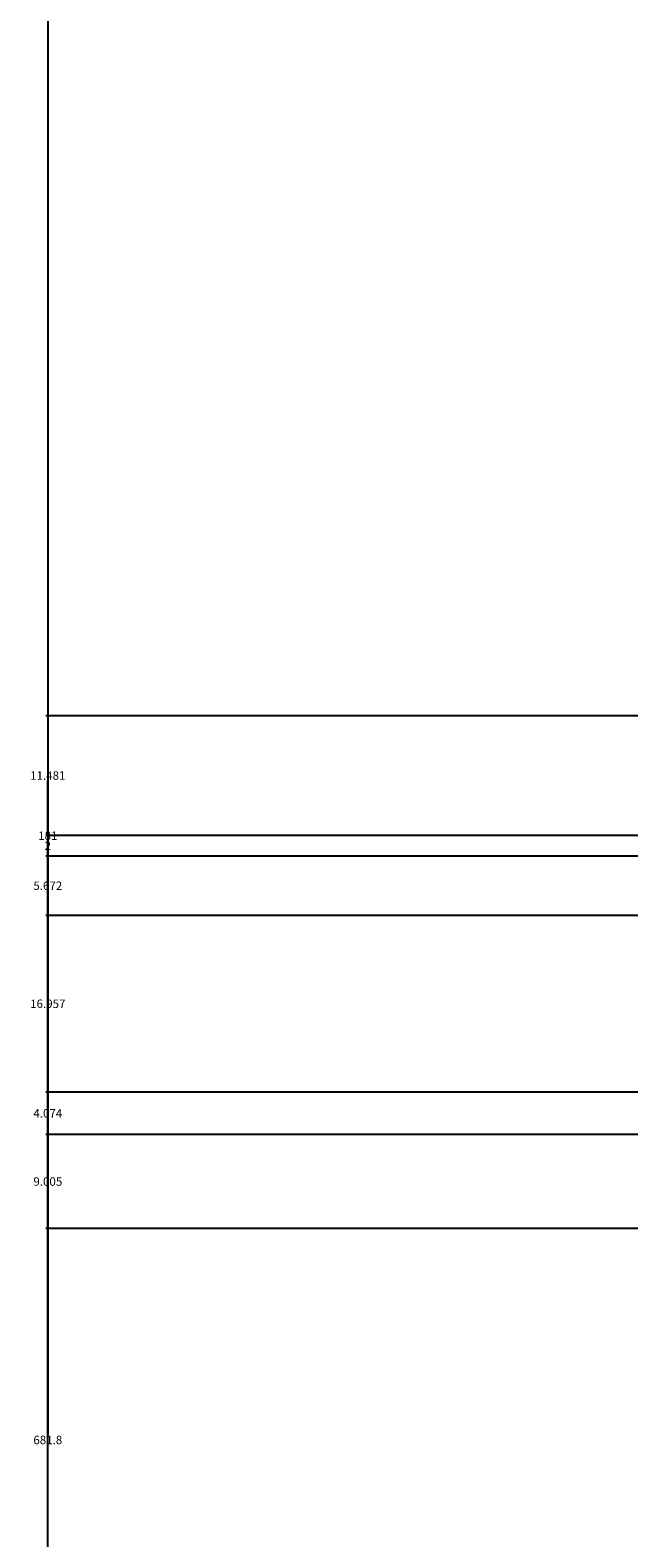
# Model space of a CAD drawing. Units: inches. Extents: x 36 to 594, y 79 to 831.
# Tile 16 of 30: x 36 to 93, y 446 to 590. Entities that reach past the tile are written whole.
import ezdxf

# ---------------------------------------------------------------- set-up
doc = ezdxf.new("R2010")
doc.units = ezdxf.units.IN
doc.header["$MEASUREMENT"] = 0
doc.layers.add('A-ANNO-DIMS', color=2, linetype='Continuous', lineweight=18)
doc.styles.get("Standard").update_dxf_attribs({"font": 'arial.ttf'})
doc.dimstyles.get("Standard").update_dxf_attribs({"dimtxt": 0.8125, "dimasz": 0.18, "dimexe": 0.18, "dimexo": 0.0625, "dimgap": 0.09, "dimtad": 0, "dimtih": 1, "dimtoh": 1, "dimdec": 4, "dimzin": 0, "dimdsep": 46, "dimlunit": 4, "dimtxsty": 'Standard', "dimcen": 0.09, "dimadec": 0, "dimazin": 0, "dimtfac": 1, "dimtdec": 4, "dimtofl": 0, "dimtmove": 0, "dimatfit": 3, "dimfxl": 1, "dimtolj": 1, "dimtzin": 0, "dimarcsym": 0})

# ---------------------------------------------------------------- blocks, each defined once
blk = doc.blocks.new('*D28')
at = {"layer": 'A-ANNO-DIMS', "color": 0, "lineweight": -2, "transparency": 16777216}
for p, q in [((269.3, 796.05), (37.49, 796.05)), ((37.67, 795.87), (37.67, 455.63)), ((37.67, 114.39), (37.67, 454.62)), ((94.8, 114.21), (37.49, 114.21))]:
    blk.add_line(p, q, dxfattribs=at)
at = {"layer": 'A-ANNO-DIMS', "color": 0, "transparency": 16777216}
for points in [[(37.64, 795.87), (37.7, 795.87), (37.67, 796.05)], [(37.64, 114.39), (37.7, 114.39), (37.67, 114.21)]]:
    blk.add_solid(points, dxfattribs=at)
at = {"layer": 'Defpoints', "color": 0, "transparency": 16777216}
for p in [(37.67, 796.05), (269.36, 796.05), (94.87, 114.21)]:
    blk.add_point(p, dxfattribs=at)
at = {"layer": 'A-ANNO-DIMS', "color": 0, "transparency": 16777216, "insert": (37.67, 455.13), "char_height": 0.812, "attachment_point": 5}
blk.add_mtext('\\A1;681.8', dxfattribs=at)
blk = doc.blocks.new('*D44')
at = {"layer": 'A-ANNO-DIMS', "color": 0, "lineweight": -2, "transparency": 16777216}
for p, q in [((72.11, 603.6), (37.49, 603.6)), ((37.67, 603.42), (37.67, 513.6)), ((37.67, 422.77), (37.67, 512.59)), ((72.11, 422.59), (37.49, 422.59))]:
    blk.add_line(p, q, dxfattribs=at)
at = {"layer": 'A-ANNO-DIMS', "color": 0, "transparency": 16777216}
for points in [[(37.64, 603.42), (37.7, 603.42), (37.67, 603.6)], [(37.64, 422.77), (37.7, 422.77), (37.67, 422.59)]]:
    blk.add_solid(points, dxfattribs=at)
at = {"layer": 'Defpoints', "color": 0, "transparency": 16777216}
for p in [(37.67, 603.6), (72.17, 603.6), (72.17, 422.59)]:
    blk.add_point(p, dxfattribs=at)
at = {"layer": 'A-ANNO-DIMS', "color": 0, "transparency": 16777216, "insert": (37.67, 513.09), "char_height": 0.812, "attachment_point": 5}
blk.add_mtext('\\A1;181', dxfattribs=at)
blk = doc.blocks.new('*D99')
at = {"layer": 'A-ANNO-DIMS', "color": 0, "lineweight": -2, "transparency": 16777216}
for p, q in [((236.23, 484.42), (37.49, 484.42)), ((37.67, 484.24), (37.67, 480.42)), ((37.67, 475.59), (37.67, 479.41)), ((232.76, 475.41), (37.49, 475.41))]:
    blk.add_line(p, q, dxfattribs=at)
at = {"layer": 'A-ANNO-DIMS', "color": 0, "transparency": 16777216}
for points in [[(37.64, 484.24), (37.7, 484.24), (37.67, 484.42)], [(37.64, 475.59), (37.7, 475.59), (37.67, 475.41)]]:
    blk.add_solid(points, dxfattribs=at)
at = {"layer": 'Defpoints', "color": 0, "transparency": 16777216}
for p in [(37.67, 484.42), (236.29, 484.42), (232.82, 475.41)]:
    blk.add_point(p, dxfattribs=at)
at = {"layer": 'A-ANNO-DIMS', "color": 0, "transparency": 16777216, "insert": (37.67, 479.92), "char_height": 0.812, "attachment_point": 5}
blk.add_mtext('\\A1;9.005', dxfattribs=at)
blk = doc.blocks.new('*D100')
at = {"layer": 'A-ANNO-DIMS', "color": 0, "lineweight": -2, "transparency": 16777216}
for p, q in [((236.23, 488.49), (37.49, 488.49)), ((37.67, 488.31), (37.67, 486.96)), ((37.67, 484.6), (37.67, 485.95)), ((236.23, 484.42), (37.49, 484.42))]:
    blk.add_line(p, q, dxfattribs=at)
at = {"layer": 'A-ANNO-DIMS', "color": 0, "transparency": 16777216}
for points in [[(37.64, 488.31), (37.7, 488.31), (37.67, 488.49)], [(37.64, 484.6), (37.7, 484.6), (37.67, 484.42)]]:
    blk.add_solid(points, dxfattribs=at)
at = {"layer": 'Defpoints', "color": 0, "transparency": 16777216}
for p in [(37.67, 488.49), (236.29, 488.49), (236.29, 484.42)]:
    blk.add_point(p, dxfattribs=at)
at = {"layer": 'A-ANNO-DIMS', "color": 0, "transparency": 16777216, "insert": (37.67, 486.46), "char_height": 0.812, "attachment_point": 5}
blk.add_mtext('\\A1;4.074', dxfattribs=at)
blk = doc.blocks.new('*D101')
at = {"layer": 'A-ANNO-DIMS', "color": 0, "lineweight": -2, "transparency": 16777216}
for p, q in [((236.23, 505.45), (37.49, 505.45)), ((37.67, 505.27), (37.67, 497.48)), ((37.67, 488.67), (37.67, 496.47)), ((236.23, 488.49), (37.49, 488.49))]:
    blk.add_line(p, q, dxfattribs=at)
at = {"layer": 'A-ANNO-DIMS', "color": 0, "transparency": 16777216}
for points in [[(37.64, 505.27), (37.7, 505.27), (37.67, 505.45)], [(37.64, 488.67), (37.7, 488.67), (37.67, 488.49)]]:
    blk.add_solid(points, dxfattribs=at)
at = {"layer": 'Defpoints', "color": 0, "transparency": 16777216}
for p in [(37.67, 505.45), (236.29, 505.45), (236.29, 488.49)]:
    blk.add_point(p, dxfattribs=at)
at = {"layer": 'A-ANNO-DIMS', "color": 0, "transparency": 16777216, "insert": (37.67, 496.97), "char_height": 0.812, "attachment_point": 5}
blk.add_mtext('\\A1;16.957', dxfattribs=at)
blk = doc.blocks.new('*D102')
at = {"layer": 'A-ANNO-DIMS', "color": 0, "lineweight": -2, "transparency": 16777216}
for p, q in [((232.76, 511.12), (37.49, 511.12)), ((37.67, 510.94), (37.67, 508.79)), ((37.67, 505.63), (37.67, 507.78)), ((236.23, 505.45), (37.49, 505.45))]:
    blk.add_line(p, q, dxfattribs=at)
at = {"layer": 'A-ANNO-DIMS', "color": 0, "transparency": 16777216}
for points in [[(37.64, 510.94), (37.7, 510.94), (37.67, 511.12)], [(37.64, 505.63), (37.7, 505.63), (37.67, 505.45)]]:
    blk.add_solid(points, dxfattribs=at)
at = {"layer": 'Defpoints', "color": 0, "transparency": 16777216}
for p in [(37.67, 511.12), (232.82, 511.12), (236.29, 505.45)]:
    blk.add_point(p, dxfattribs=at)
at = {"layer": 'A-ANNO-DIMS', "color": 0, "transparency": 16777216, "insert": (37.67, 508.29), "char_height": 0.812, "attachment_point": 5}
blk.add_mtext('\\A1;5.672', dxfattribs=at)
blk = doc.blocks.new('*D103')
at = {"layer": 'A-ANNO-DIMS', "color": 0, "lineweight": -2, "transparency": 16777216}
for p, q in [((232.76, 513.12), (37.49, 513.12)), ((37.67, 512.94), (37.67, 512.62)), ((232.76, 511.12), (37.49, 511.12)), ((37.67, 511.3), (37.67, 511.62))]:
    blk.add_line(p, q, dxfattribs=at)
at = {"layer": 'A-ANNO-DIMS', "color": 0, "transparency": 16777216}
for points in [[(37.64, 512.94), (37.7, 512.94), (37.67, 513.12)], [(37.64, 511.3), (37.7, 511.3), (37.67, 511.12)]]:
    blk.add_solid(points, dxfattribs=at)
at = {"layer": 'Defpoints', "color": 0, "transparency": 16777216}
for p in [(37.67, 513.12), (232.82, 513.12), (232.82, 511.12)]:
    blk.add_point(p, dxfattribs=at)
at = {"layer": 'A-ANNO-DIMS', "color": 0, "transparency": 16777216, "insert": (37.67, 512.12), "char_height": 0.812, "attachment_point": 5}
blk.add_mtext('\\A1;2', dxfattribs=at)
blk = doc.blocks.new('*D104')
at = {"layer": 'A-ANNO-DIMS', "color": 0, "lineweight": -2, "transparency": 16777216}
for p, q in [((232.76, 524.6), (37.49, 524.6)), ((37.67, 524.42), (37.67, 519.37)), ((37.67, 513.3), (37.67, 518.36)), ((232.76, 513.12), (37.49, 513.12))]:
    blk.add_line(p, q, dxfattribs=at)
at = {"layer": 'A-ANNO-DIMS', "color": 0, "transparency": 16777216}
for points in [[(37.64, 524.42), (37.7, 524.42), (37.67, 524.6)], [(37.64, 513.3), (37.7, 513.3), (37.67, 513.12)]]:
    blk.add_solid(points, dxfattribs=at)
at = {"layer": 'Defpoints', "color": 0, "transparency": 16777216}
for p in [(37.67, 524.6), (232.82, 524.6), (232.82, 513.12)]:
    blk.add_point(p, dxfattribs=at)
at = {"layer": 'A-ANNO-DIMS', "color": 0, "transparency": 16777216, "insert": (37.67, 518.86), "char_height": 0.812, "attachment_point": 5}
blk.add_mtext('\\A1;11.481', dxfattribs=at)

msp = doc.modelspace()

# ---------------------------------------------------------------- dimensions: what is measured, and where the dimension line sits
at = {"layer": 'A-ANNO-DIMS'}
for base, p1, p2, override, picture, middle in [((37.6733, 796.0465), (94.8658, 114.2124), (269.3592, 796.0465), {"dimdec": 1, "dimlfac": 1, "dimrnd": 0, "dimzin": 0, "dimdsep": 46, "dimlunit": 2}, '*D28', (37.6733, 455.1294)), ((37.6733, 603.598), (72.1733, 422.5882), (72.1733, 603.598), {"dimdec": 0, "dimlfac": 1, "dimrnd": 0, "dimzin": 0, "dimdsep": 46, "dimlunit": 2}, '*D44', (37.6733, 513.0931)), ((37.6733, 524.6037), (232.8216, 513.1224), (232.8216, 524.6037), {"dimdec": 3, "dimlfac": 1, "dimrnd": 0, "dimzin": 0, "dimdsep": 46, "dimlunit": 2}, '*D104', (37.6733, 518.863)), ((37.6733, 513.1224), (232.8216, 511.1224), (232.8216, 513.1224), {"dimdec": 0, "dimlfac": 1, "dimrnd": 0, "dimzin": 0, "dimdsep": 46, "dimlunit": 2}, '*D103', (37.6733, 512.1224)), ((37.67335, 511.12236), (236.29105, 505.44988), (232.82156, 511.12236), {"dimdec": 3, "dimlfac": 1, "dimrnd": 0, "dimzin": 0, "dimdsep": 46, "dimlunit": 2}, '*D102', (37.67335, 508.28612)), ((37.6733, 505.4499), (236.2911, 488.4928), (236.2911, 505.4499), {"dimdec": 3, "dimlfac": 1, "dimrnd": 0, "dimzin": 0, "dimdsep": 46, "dimlunit": 2}, '*D101', (37.6733, 496.9714)), ((37.6733, 488.4928), (236.2911, 484.4187), (236.2911, 488.4928), {"dimdec": 3, "dimlfac": 1, "dimrnd": 0, "dimzin": 0, "dimdsep": 46, "dimlunit": 2}, '*D100', (37.6733, 486.4558)), ((37.6733, 484.4187), (232.8216, 475.4136), (236.2911, 484.4187), {"dimdec": 3, "dimlfac": 1, "dimrnd": 0, "dimzin": 0, "dimdsep": 46, "dimlunit": 2}, '*D99', (37.6733, 479.9162))]:
    dim = msp.add_linear_dim(base=base, p1=p1, p2=p2, angle=90, dimstyle='Standard', override=override, dxfattribs=at)
    dim.commit()
    dim.dimension.update_dxf_attribs({"geometry": picture, "text_midpoint": middle})

doc.saveas('drawing.dxf')
